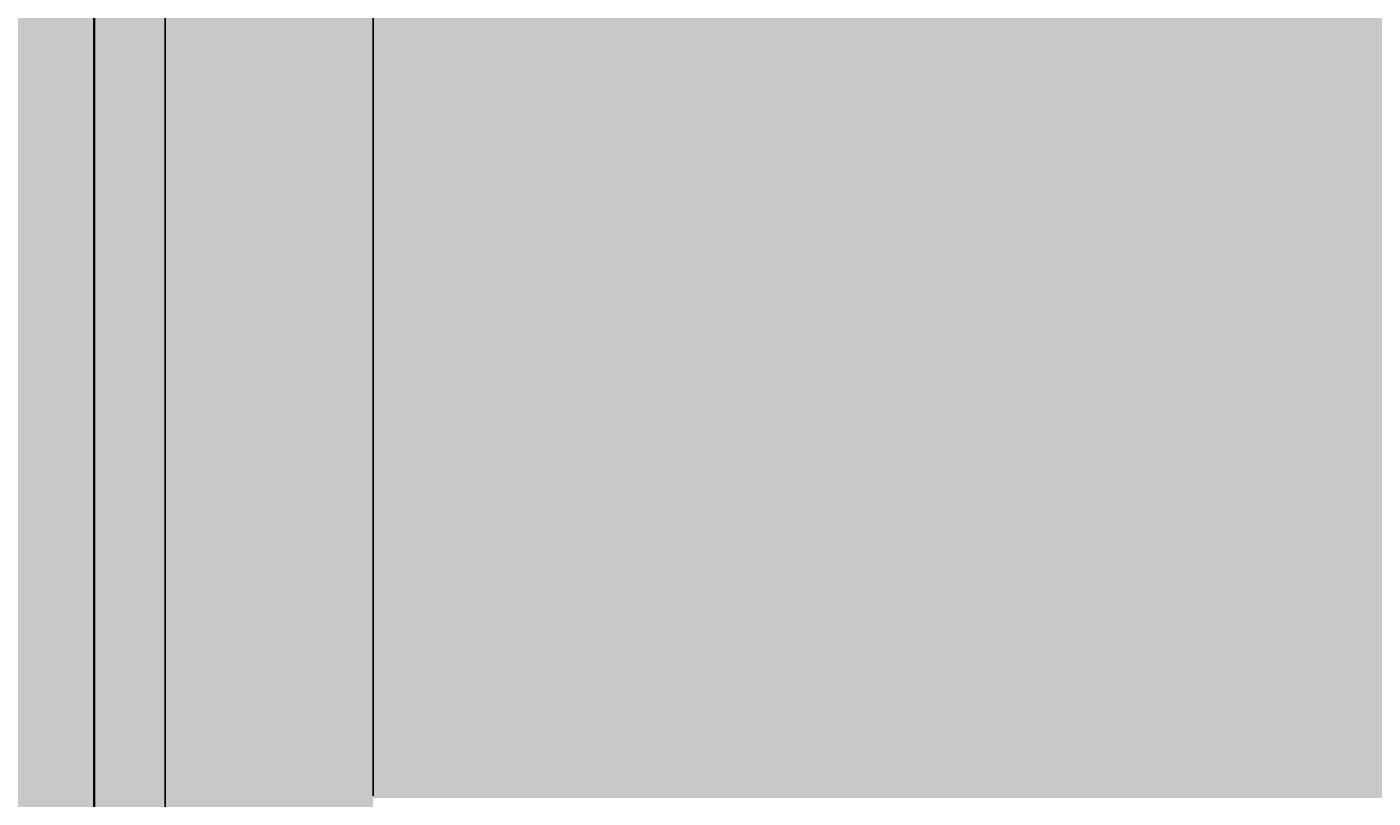
# Model space of a CAD drawing. Units: feet. Extents: x 2695 to 2912, y 795 to 1139.
# Tile 65 of 83: x 2769 to 2805, y 1021 to 1041. Entities that reach past the tile are written whole.
import ezdxf

# ---------------------------------------------------------------- set-up
doc = ezdxf.new("R2010")
doc.units = ezdxf.units.FT
for name, color, linetype, lineweight in [('A-ANNO-DIMS', 2, 'Continuous', 18), ('A-ELEV', 7, 'Continuous', 35), ('A-ELEV-PATT', 252, 'Continuous', 13)]:
    doc.layers.add(name, color=color, linetype=linetype, lineweight=lineweight)
doc.styles.get("Standard").update_dxf_attribs({"font": 'arial.ttf'})
doc.dimstyles.get("Standard").update_dxf_attribs({"dimtxt": 0.18, "dimasz": 0.18, "dimexe": 0.18, "dimexo": 0.0625, "dimgap": 0.09, "dimtad": 0, "dimtih": 1, "dimtoh": 1, "dimdec": 1, "dimzin": 0, "dimdsep": 46, "dimlunit": 3, "dimtxsty": 'Standard', "dimcen": 0.09, "dimadec": 0, "dimazin": 0, "dimtfac": 1, "dimtdec": 1, "dimtofl": 0, "dimtmove": 0, "dimatfit": 3, "dimfxl": 1, "dimtolj": 1, "dimtzin": 0, "dimarcsym": 0})

# ---------------------------------------------------------------- blocks, each defined once
blk = doc.blocks.new('*D9')
at = {"layer": 'A-ANNO-DIMS', "color": 0, "lineweight": -2, "transparency": 16777216}
for p, q in [((2770.636, 1122.993), (2770.636, 1138.886)), ((2770.816, 1138.706), (2773.942, 1138.706)), ((2777.854, 1138.706), (2774.728, 1138.706)), ((2778.034, 1020.886), (2778.034, 1138.886))]:
    blk.add_line(p, q, dxfattribs=at)
at = {"layer": 'A-ANNO-DIMS', "color": 0, "transparency": 16777216}
for points in [[(2770.816, 1138.736), (2770.816, 1138.676), (2770.636, 1138.706)], [(2777.854, 1138.736), (2777.854, 1138.676), (2778.034, 1138.706)]]:
    blk.add_solid(points, dxfattribs=at)
at = {"layer": 'Defpoints', "color": 0, "transparency": 16777216}
for p in [(2778.034, 1138.706), (2770.636, 1122.931), (2778.034, 1020.824)]:
    blk.add_point(p, dxfattribs=at)
at = {"layer": 'A-ANNO-DIMS', "color": 0, "transparency": 16777216, "insert": (2774.335, 1138.706), "char_height": 0.18, "attachment_point": 5}
blk.add_mtext('\\A1;7.398', dxfattribs=at)
blk = doc.blocks.new('*D10')
at = {"layer": 'A-ANNO-DIMS', "color": 0, "lineweight": -2, "transparency": 16777216}
for p, q in [((2778.034, 1020.886), (2778.034, 1138.886)), ((2778.214, 1138.706), (2810.411, 1138.706)), ((2843.395, 1138.706), (2811.198, 1138.706)), ((2843.575, 1020.886), (2843.575, 1138.886))]:
    blk.add_line(p, q, dxfattribs=at)
at = {"layer": 'A-ANNO-DIMS', "color": 0, "transparency": 16777216}
for points in [[(2778.214, 1138.736), (2778.214, 1138.676), (2778.034, 1138.706)], [(2843.395, 1138.736), (2843.395, 1138.676), (2843.575, 1138.706)]]:
    blk.add_solid(points, dxfattribs=at)
at = {"layer": 'Defpoints', "color": 0, "transparency": 16777216}
for p in [(2843.575, 1138.706), (2778.034, 1020.824), (2843.575, 1020.824)]:
    blk.add_point(p, dxfattribs=at)
at = {"layer": 'A-ANNO-DIMS', "color": 0, "transparency": 16777216, "insert": (2810.805, 1138.706), "char_height": 0.18, "attachment_point": 5}
blk.add_mtext('\\A1;65.54', dxfattribs=at)
blk = doc.blocks.new('*D48')
at = {"layer": 'A-ANNO-DIMS', "color": 0, "lineweight": -2, "transparency": 16777216}
for p, q in [((2770.636, 972.03), (2770.636, 1138.886)), ((2770.816, 1138.706), (2771.263, 1138.706)), ((2772.342, 1138.706), (2771.894, 1138.706)), ((2772.522, 972.03), (2772.522, 1138.886))]:
    blk.add_line(p, q, dxfattribs=at)
at = {"layer": 'A-ANNO-DIMS', "color": 0, "transparency": 16777216}
for points in [[(2770.816, 1138.736), (2770.816, 1138.676), (2770.636, 1138.706)], [(2772.342, 1138.736), (2772.342, 1138.676), (2772.522, 1138.706)]]:
    blk.add_solid(points, dxfattribs=at)
at = {"layer": 'Defpoints', "color": 0, "transparency": 16777216}
for p in [(2772.522, 1138.706), (2770.636, 971.967), (2772.522, 971.967)]:
    blk.add_point(p, dxfattribs=at)
at = {"layer": 'A-ANNO-DIMS', "color": 0, "transparency": 16777216, "insert": (2771.579, 1138.706), "char_height": 0.18, "attachment_point": 5}
blk.add_mtext('\\A1;1.89', dxfattribs=at)
blk = doc.blocks.new('*D49')
at = {"layer": 'A-ANNO-DIMS', "color": 0, "lineweight": -2, "transparency": 16777216}
for p, q in [((2772.522, 972.03), (2772.522, 1138.886)), ((2772.702, 1138.706), (2790.888, 1138.706)), ((2809.861, 1138.706), (2791.674, 1138.706)), ((2810.041, 972.03), (2810.041, 1138.886))]:
    blk.add_line(p, q, dxfattribs=at)
at = {"layer": 'A-ANNO-DIMS', "color": 0, "transparency": 16777216}
for points in [[(2772.702, 1138.736), (2772.702, 1138.676), (2772.522, 1138.706)], [(2809.861, 1138.736), (2809.861, 1138.676), (2810.041, 1138.706)]]:
    blk.add_solid(points, dxfattribs=at)
at = {"layer": 'Defpoints', "color": 0, "transparency": 16777216}
for p in [(2810.041, 1138.706), (2772.522, 971.967), (2810.041, 971.967)]:
    blk.add_point(p, dxfattribs=at)
at = {"layer": 'A-ANNO-DIMS', "color": 0, "transparency": 16777216, "insert": (2791.281, 1138.706), "char_height": 0.18, "attachment_point": 5}
blk.add_mtext('\\A1;37.52', dxfattribs=at)

msp = doc.modelspace()

# ---------------------------------------------------------------- hatches: boundary and pattern name
at = {"layer": 'A-ELEV-PATT'}
h = msp.add_hatch(color=256, dxfattribs=at)
h.set_gradient(color1=(147, 149, 152), color2=(147, 149, 152), tint=1)
h.paths.add_polyline_path([(2770.6361, 1118.4096), (2710.6361, 1118.4096), (2710.6361, 1062.9306), (2770.6361, 1062.9306)])
h.paths.add_polyline_path([(2890.6361, 1103.3378), (2770.6361, 1103.3378), (2770.6361, 1062.9306), (2890.6361, 1062.9306)])
h.paths.add_polyline_path([(2730.7081, 1048.1052), (2755.1125, 1048.1052), (2755.1125, 936.9306), (2770.6361, 936.9306), (2770.6361, 1050.3105), (2715.8852, 1050.3105), (2715.8852, 936.9306), (2730.7081, 936.9306)])
h.paths.add_polyline_path([(2890.6361, 1050.3105), (2770.6361, 1050.3105), (2770.6361, 971.9673), (2778.0341, 971.9673), (2778.0341, 1020.8235), (2843.575, 1020.8235), (2843.575, 971.9673), (2890.6361, 971.9673)])
h.paths.add_polyline_path([(2888.1882, 970.7156), (2843.575, 970.7156), (2843.575, 964.8267), (2888.1882, 964.8267)])
h.paths.add_polyline_path([(2888.1882, 964.1328), (2843.575, 964.1328), (2843.575, 956.614), (2888.1882, 956.614)])
h.paths.add_polyline_path([(2888.1882, 955.9202), (2843.575, 955.9202), (2843.575, 949.2892), (2888.1882, 949.2892)])
h.paths.add_polyline_path([(2888.1882, 948.5954), (2843.575, 948.5954), (2843.575, 941.3507), (2888.1882, 941.3507)])
h.paths.add_polyline_path([(2888.1882, 940.6569), (2843.575, 940.6569), (2843.575, 936.9306), (2888.1882, 936.9306)])
h.paths.add_polyline_path([(2890.6361, 970.7156), (2888.9368, 970.7156), (2888.9368, 964.8267), (2890.6361, 964.8267)])
h.paths.add_polyline_path([(2890.6361, 964.1328), (2888.9368, 964.1328), (2888.9368, 956.614), (2890.6361, 956.614)])
h.paths.add_polyline_path([(2890.6361, 955.9202), (2888.9368, 955.9202), (2888.9368, 949.2892), (2890.6361, 949.2892)])
h.paths.add_polyline_path([(2890.6361, 940.6569), (2888.9368, 940.6569), (2888.9368, 936.9306), (2890.6361, 936.9306)])
h.paths.add_polyline_path([(2890.6361, 948.5954), (2888.9368, 948.5954), (2888.9368, 941.3507), (2890.6361, 941.3507)])
h.paths.add_polyline_path([(2772.5216, 970.7156), (2770.6361, 970.7156), (2770.6361, 964.8267), (2772.5216, 964.8267)])
h.paths.add_polyline_path([(2772.5216, 964.1328), (2770.6361, 964.1328), (2770.6361, 956.614), (2772.5216, 956.614)])
h.paths.add_polyline_path([(2772.5216, 955.9202), (2770.6361, 955.9202), (2770.6361, 949.2892), (2772.5216, 949.2892)])
h.paths.add_polyline_path([(2772.5216, 948.5954), (2770.6361, 948.5954), (2770.6361, 941.3507), (2772.5216, 941.3507)])
h.paths.add_polyline_path([(2772.5216, 940.6569), (2770.6361, 940.6569), (2770.6361, 936.9306), (2772.5216, 936.9306)])
h.paths.add_polyline_path([(2778.0341, 940.6569), (2773.2702, 940.6569), (2773.2702, 936.9306), (2778.0341, 936.9306)])
h.paths.add_polyline_path([(2778.0341, 970.7156), (2773.2702, 970.7156), (2773.2702, 964.8267), (2778.0341, 964.8267)])
h.paths.add_polyline_path([(2778.0341, 964.1328), (2773.2702, 964.1328), (2773.2702, 956.614), (2778.0341, 956.614)])
h.paths.add_polyline_path([(2778.0341, 955.9202), (2773.2702, 955.9202), (2773.2702, 949.2892), (2778.0341, 949.2892)])
h.paths.add_polyline_path([(2778.0341, 948.5954), (2773.2702, 948.5954), (2773.2702, 941.3507), (2778.0341, 941.3507)])
h.paths.add_polyline_path([(2810.0407, 940.6569), (2780.0341, 940.6569), (2780.0341, 936.9306), (2810.0407, 936.9306)])
h.paths.add_polyline_path([(2890.6361, 924.3105), (2770.6361, 924.3105), (2770.6361, 810.9306), (2773.5029, 810.9306), (2773.5029, 905.5143), (2805.9398, 905.5143), (2838.3767, 905.5143), (2838.3767, 810.9306), (2890.6361, 810.9306)])

# ---------------------------------------------------------------- linework, layer by layer
at = {"layer": 'A-ELEV'}
msp.add_line((2770.6361, 1050.3105), (2770.6361, 936.9306), dxfattribs=at)

# ---------------------------------------------------------------- dimensions: what is measured, and where the dimension line sits
at = {"layer": 'A-ANNO-DIMS'}
for base, p1, p2, override, picture, middle in [((2778.0341, 1138.7056), (2770.6361, 1122.9306), (2778.0341, 1020.8235), {"dimdec": 3, "dimlfac": 1, "dimrnd": 0, "dimzin": 0, "dimdsep": 46, "dimlunit": 2}, '*D9', (2774.3351, 1138.7056)), ((2772.5216, 1138.7056), (2770.6361, 971.9673), (2772.5216, 971.9673), {"dimdec": 2, "dimlfac": 1, "dimrnd": 0, "dimzin": 0, "dimdsep": 46, "dimlunit": 2}, '*D48', (2771.5788, 1138.7056)), ((2810.0407, 1138.7056), (2772.5216, 971.9673), (2810.0407, 971.9673), {"dimdec": 2, "dimlfac": 1, "dimrnd": 0, "dimzin": 0, "dimdsep": 46, "dimlunit": 2}, '*D49', (2791.2811, 1138.7056)), ((2843.575, 1138.7056), (2778.0341, 1020.8235), (2843.575, 1020.8235), {"dimdec": 2, "dimlfac": 1, "dimrnd": 0, "dimzin": 0, "dimdsep": 46, "dimlunit": 2}, '*D10', (2810.8045, 1138.7056))]:
    dim = msp.add_linear_dim(base=base, p1=p1, p2=p2, dimstyle='Standard', override=override, dxfattribs=at)
    dim.commit()
    dim.dimension.update_dxf_attribs({"geometry": picture, "text_midpoint": middle})

doc.saveas('drawing.dxf')
